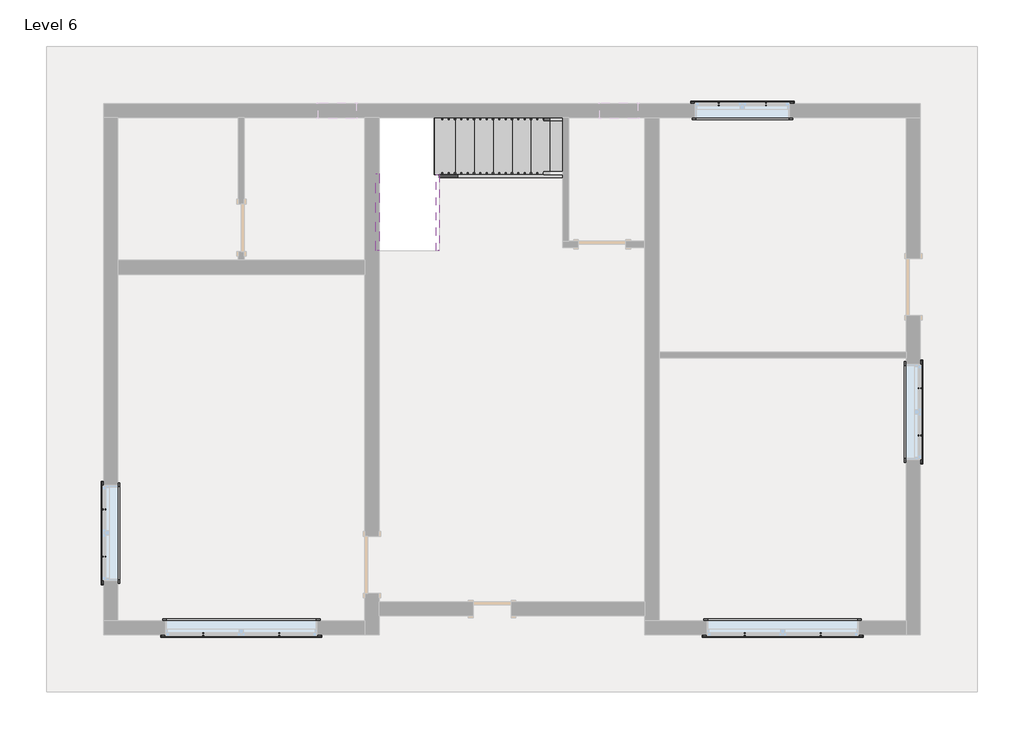
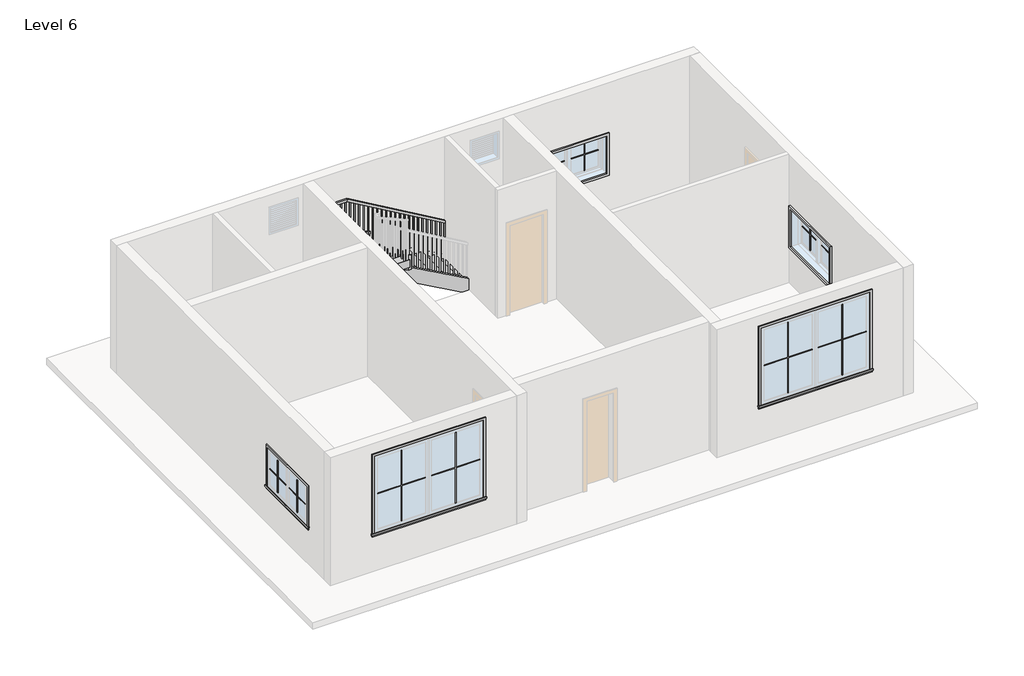
# One storey, part 2 of 2: 20 proxies, 4 members, 1 railing, 1 stair flight.
"""IFC4 building model written with IfcOpenShell, lengths in millimetres."""

from ifc_helpers import new_model, si_unit, frame, origin, place, context, project, spatial, polyline, outline, extrude, faceted_brep, transform, mapped, element, save
from components import muntin_pattern_2x2_muntin_pattern_2x2_9352d081, muntin_pattern_2x2_muntin_pattern_2x2_5c2cbe28, muntin_pattern_2x2_muntin_pattern_2x2_bb8d4d84, muntin_pattern_2x2_muntin_pattern_2x2_d03a1f3c, trim_window_exterior_flat_with_sill_979bde60, trim_window_exterior_flat_with_sill_359ed2ce, trim_window_interior_flat_picture_frame_7883d11b, trim_window_interior_flat_picture_frame_939a8053, stair_flight_d8623c0a

model = new_model("IFC4")

# Units and contexts
model_context = context("Model", 3, world=origin())
ifc_project = project(units=[si_unit("LENGTHUNIT", "METRE", prefix="MILLI")], contexts=[model_context])

# Site, building, storey
site = spatial("IfcSite", under=ifc_project)
building = spatial("IfcBuilding", under=site)
storey = spatial("IfcBuildingStorey", under=building, Name="Level 6", Elevation=15849.6)

# Proxies
placement = place(None, origin())
muntin_pattern_2x2_muntin_pattern_2x2_shape = muntin_pattern_2x2_muntin_pattern_2x2_9352d081(model_context)
element("IfcBuildingElementProxy", 1, Name="Muntin Pattern_2x2 : Muntin Pattern_2x2", ObjectType="Muntin Pattern_2x2 : Muntin Pattern_2x2", at=placement, inside=storey, context=model_context, shape_type="MappedRepresentation", body=[
    mapped(muntin_pattern_2x2_muntin_pattern_2x2_shape, transform((-7798.9165084, -1764.5743005, 16833.85), x_axis=(0.0, 1.0, 0.0), y_axis=(-1.0, 0.0, 0.0), z_axis=(0.0, 0.0, 1.0))),
])
element("IfcBuildingElementProxy", 2, Name="Muntin Pattern_2x2 : Muntin Pattern_2x2", ObjectType="Muntin Pattern_2x2 : Muntin Pattern_2x2", at=placement, inside=storey, context=model_context, shape_type="MappedRepresentation", body=[
    mapped(muntin_pattern_2x2_muntin_pattern_2x2_shape, transform((5288.4334916, 937.3506995, 16833.85), x_axis=(0.0, -1.0, 0.0), y_axis=(1.0, 0.0, 0.0), z_axis=(0.0, 0.0, 1.0))),
])
element("IfcBuildingElementProxy", 3, Name="Muntin Pattern_2x2 : Muntin Pattern_2x2", ObjectType="Muntin Pattern_2x2 : Muntin Pattern_2x2", at=placement, inside=storey, context=model_context, shape_type="MappedRepresentation", body=[
    mapped(muntin_pattern_2x2_muntin_pattern_2x2_shape, transform((2061.0459916, 5501.4131995, 16833.85), x_axis=(1.0, 0.0, 0.0), y_axis=(0.0, 1.0, 0.0), z_axis=(0.0, 0.0, 1.0))),
])
muntin_pattern_2x2_muntin_pattern_2x2_2_shape = muntin_pattern_2x2_muntin_pattern_2x2_5c2cbe28(model_context)
element("IfcBuildingElementProxy", 4, Name="Muntin Pattern_2x2 : Muntin Pattern_2x2", ObjectType="Muntin Pattern_2x2 : Muntin Pattern_2x2", at=placement, inside=storey, context=model_context, shape_type="MappedRepresentation", body=[
    mapped(muntin_pattern_2x2_muntin_pattern_2x2_2_shape, transform((-7798.9165084, -1005.7493005, 16833.85), x_axis=(0.0, -1.0, 0.0), y_axis=(1.0, 0.0, 0.0), z_axis=(0.0, 0.0, 1.0))),
])
element("IfcBuildingElementProxy", 5, Name="Muntin Pattern_2x2 : Muntin Pattern_2x2", ObjectType="Muntin Pattern_2x2 : Muntin Pattern_2x2", at=placement, inside=storey, context=model_context, shape_type="MappedRepresentation", body=[
    mapped(muntin_pattern_2x2_muntin_pattern_2x2_2_shape, transform((5288.4334916, 178.5256995, 16833.85), x_axis=(0.0, 1.0, 0.0), y_axis=(-1.0, 0.0, 0.0), z_axis=(0.0, 0.0, 1.0))),
])
element("IfcBuildingElementProxy", 6, Name="Muntin Pattern_2x2 : Muntin Pattern_2x2", ObjectType="Muntin Pattern_2x2 : Muntin Pattern_2x2", at=placement, inside=storey, context=model_context, shape_type="MappedRepresentation", body=[
    mapped(muntin_pattern_2x2_muntin_pattern_2x2_2_shape, transform((2819.8709916, 5501.4131995, 16833.85), x_axis=(-1.0, 0.0, 0.0), y_axis=(0.0, -1.0, 0.0), z_axis=(0.0, 0.0, 1.0))),
])
muntin_pattern_2x2_muntin_pattern_2x2_3_shape = muntin_pattern_2x2_muntin_pattern_2x2_bb8d4d84(model_context)
element("IfcBuildingElementProxy", 7, Name="Muntin Pattern_2x2 : Muntin Pattern_2x2", ObjectType="Muntin Pattern_2x2 : Muntin Pattern_2x2", at=placement, inside=storey, context=model_context, shape_type="MappedRepresentation", body=[
    mapped(muntin_pattern_2x2_muntin_pattern_2x2_3_shape, transform((-4990.6290084, -3013.9368005, 16833.85), x_axis=(-1.0, 0.0, 0.0), y_axis=(0.0, -1.0, 0.0), z_axis=(0.0, 0.0, 1.0))),
])
element("IfcBuildingElementProxy", 8, Name="Muntin Pattern_2x2 : Muntin Pattern_2x2", ObjectType="Muntin Pattern_2x2 : Muntin Pattern_2x2", at=placement, inside=storey, context=model_context, shape_type="MappedRepresentation", body=[
    mapped(muntin_pattern_2x2_muntin_pattern_2x2_3_shape, transform((3696.1709916, -3013.9368005, 16833.85), x_axis=(-1.0, 0.0, 0.0), y_axis=(0.0, -1.0, 0.0), z_axis=(0.0, 0.0, 1.0))),
])
muntin_pattern_2x2_muntin_pattern_2x2_4_shape = muntin_pattern_2x2_muntin_pattern_2x2_d03a1f3c(model_context)
element("IfcBuildingElementProxy", 9, Name="Muntin Pattern_2x2 : Muntin Pattern_2x2", ObjectType="Muntin Pattern_2x2 : Muntin Pattern_2x2", at=placement, inside=storey, context=model_context, shape_type="MappedRepresentation", body=[
    mapped(muntin_pattern_2x2_muntin_pattern_2x2_4_shape, transform((-6206.6540084, -3013.9368005, 16833.85), x_axis=(1.0, 0.0, 0.0), y_axis=(0.0, 1.0, 0.0), z_axis=(0.0, 0.0, 1.0))),
])
element("IfcBuildingElementProxy", 10, Name="Muntin Pattern_2x2 : Muntin Pattern_2x2", ObjectType="Muntin Pattern_2x2 : Muntin Pattern_2x2", at=placement, inside=storey, context=model_context, shape_type="MappedRepresentation", body=[
    mapped(muntin_pattern_2x2_muntin_pattern_2x2_4_shape, transform((2480.1459916, -3013.9368005, 16833.85), x_axis=(1.0, 0.0, 0.0), y_axis=(0.0, 1.0, 0.0), z_axis=(0.0, 0.0, 1.0))),
])
trim_window_exterior_flat_with_sill_shape = trim_window_exterior_flat_with_sill_979bde60(model_context)
element("IfcBuildingElementProxy", 11, Name="Trim-Window-Exterior-Flat : with Sill", ObjectType="Trim-Window-Exterior-Flat : with Sill", at=placement, inside=storey, context=model_context, shape_type="MappedRepresentation", body=[
    mapped(trim_window_exterior_flat_with_sill_shape, transform((-7808.4415084, -1385.1618005, 17678.4), x_axis=(0.0, -1.0, 0.0), y_axis=(0.0, 0.0, 1.0), z_axis=(-1.0, 0.0, 0.0))),
])
element("IfcBuildingElementProxy", 12, Name="Trim-Window-Exterior-Flat : with Sill", ObjectType="Trim-Window-Exterior-Flat : with Sill", at=placement, inside=storey, context=model_context, shape_type="MappedRepresentation", body=[
    mapped(trim_window_exterior_flat_with_sill_shape, transform((5297.9584916, 557.9381995, 17678.4), x_axis=(0.0, 1.0, 0.0), y_axis=(0.0, 0.0, 1.0), z_axis=(1.0, 0.0, 0.0))),
])
element("IfcBuildingElementProxy", 13, Name="Trim-Window-Exterior-Flat : with Sill", ObjectType="Trim-Window-Exterior-Flat : with Sill", at=placement, inside=storey, context=model_context, shape_type="MappedRepresentation", body=[
    mapped(trim_window_exterior_flat_with_sill_shape, transform((2440.4584916, 5510.9381995, 17678.4), x_axis=(-1.0, 0.0, 0.0), y_axis=(0.0, 0.0, 1.0), z_axis=(0.0, 1.0, 0.0))),
])
trim_window_exterior_flat_with_sill_2_shape = trim_window_exterior_flat_with_sill_359ed2ce(model_context)
element("IfcBuildingElementProxy", 14, Name="Trim-Window-Exterior-Flat : with Sill", ObjectType="Trim-Window-Exterior-Flat : with Sill", at=placement, inside=storey, context=model_context, shape_type="MappedRepresentation", body=[
    mapped(trim_window_exterior_flat_with_sill_2_shape, transform((-5598.6415084, -3023.4618005, 18592.8), x_axis=(1.0, 0.0, 0.0), y_axis=(0.0, 0.0, 1.0), z_axis=(0.0, -1.0, 0.0))),
])
element("IfcBuildingElementProxy", 15, Name="Trim-Window-Exterior-Flat : with Sill", ObjectType="Trim-Window-Exterior-Flat : with Sill", at=placement, inside=storey, context=model_context, shape_type="MappedRepresentation", body=[
    mapped(trim_window_exterior_flat_with_sill_2_shape, transform((3088.1584916, -3023.4618005, 18592.8), x_axis=(1.0, 0.0, 0.0), y_axis=(0.0, 0.0, 1.0), z_axis=(0.0, -1.0, 0.0))),
])
trim_window_interior_flat_picture_frame_shape = trim_window_interior_flat_picture_frame_7883d11b(model_context)
element("IfcBuildingElementProxy", 16, Name="Trim-Window-Interior-Flat : Picture Frame", ObjectType="Trim-Window-Interior-Flat : Picture Frame", at=placement, inside=storey, context=model_context, shape_type="MappedRepresentation", body=[
    mapped(trim_window_interior_flat_picture_frame_shape, transform((-7579.8415084, -1385.1618005, 17678.4), x_axis=(0.0, 1.0, 0.0), y_axis=(0.0, 0.0, 1.0), z_axis=(1.0, 0.0, 0.0))),
])
element("IfcBuildingElementProxy", 17, Name="Trim-Window-Interior-Flat : Picture Frame", ObjectType="Trim-Window-Interior-Flat : Picture Frame", at=placement, inside=storey, context=model_context, shape_type="MappedRepresentation", body=[
    mapped(trim_window_interior_flat_picture_frame_shape, transform((5069.3584916, 557.9381995, 17678.4), x_axis=(0.0, -1.0, 0.0), y_axis=(0.0, 0.0, 1.0), z_axis=(-1.0, 0.0, 0.0))),
])
element("IfcBuildingElementProxy", 18, Name="Trim-Window-Interior-Flat : Picture Frame", ObjectType="Trim-Window-Interior-Flat : Picture Frame", at=placement, inside=storey, context=model_context, shape_type="MappedRepresentation", body=[
    mapped(trim_window_interior_flat_picture_frame_shape, transform((2440.4584916, 5282.3381995, 17678.4), x_axis=(1.0, 0.0, 0.0), y_axis=(0.0, 0.0, 1.0), z_axis=(0.0, -1.0, 0.0))),
])
trim_window_interior_flat_picture_frame_2_shape = trim_window_interior_flat_picture_frame_939a8053(model_context)
element("IfcBuildingElementProxy", 19, Name="Trim-Window-Interior-Flat : Picture Frame", ObjectType="Trim-Window-Interior-Flat : Picture Frame", at=placement, inside=storey, context=model_context, shape_type="MappedRepresentation", body=[
    mapped(trim_window_interior_flat_picture_frame_2_shape, transform((-5598.6415084, -2794.8618005, 18592.8), x_axis=(-1.0, 0.0, 0.0), y_axis=(0.0, 0.0, 1.0), z_axis=(0.0, 1.0, 0.0))),
])
element("IfcBuildingElementProxy", 20, Name="Trim-Window-Interior-Flat : Picture Frame", ObjectType="Trim-Window-Interior-Flat : Picture Frame", at=placement, inside=storey, context=model_context, shape_type="MappedRepresentation", body=[
    mapped(trim_window_interior_flat_picture_frame_2_shape, transform((3088.1584916, -2794.8618005, 18592.8), x_axis=(-1.0, 0.0, 0.0), y_axis=(0.0, 0.0, 1.0), z_axis=(0.0, 1.0, 0.0))),
])

# Members
element("IfcMember", 21, ObjectType="Stringer - 2\" Width", at=placement, inside=storey, context=model_context, shape_type="SweptSolid", body=[
    extrude(outline(polyline([(15849.6, -442.4415084), (16113.6428392, -442.4415084), (17214.3095059, -2423.6415084), (16865.6308318, -2423.6415084), (15849.6, -594.7860112), (15849.6, -442.4415084)])), frame((0.0, 4317.5146777, 0.0), z_axis=(0.0, 1.0, 0.0), x_axis=(0.0, 0.0, 1.0)), (0.0, 0.0, 1.0), 50.8),
])
element("IfcMember", 22, ObjectType="Stringer - 2\" Width", at=placement, inside=storey, context=model_context, shape_type="SweptSolid", body=[
    extrude(outline(polyline([(4368.3146777, 17411.845537), (4368.3146777, 17063.2006925), (3148.7383287, 17740.4643411), (3148.7383287, 18089.1091856), (4368.3146777, 17411.845537)])), frame((-2474.4415084, 0.0, 0.0), z_axis=(1.0, 0.0, 0.0), x_axis=(0.0, 1.0, 0.0)), (0.0, 0.0, 1.0), 50.8),
])
element("IfcMember", 23, ObjectType="Stringer - 2\" Width", at=placement, inside=storey, context=model_context, shape_type="SweptSolid", body=[
    extrude(outline(polyline([(15849.6, -442.4415084), (16113.6428392, -442.4415084), (16904.2636166, -1865.5589077), (16904.2636166, -2493.1805211), (15849.6, -594.7860112), (15849.6, -442.4415084)])), frame((0.0, 5282.3381995, 0.0), z_axis=(0.0, 1.0, 0.0), x_axis=(0.0, 0.0, 1.0)), (0.0, 0.0, 1.0), 50.8),
])
element("IfcMember", 24, ObjectType="Stringer - 2\" Width", at=placement, inside=storey, context=model_context, shape_type="SweptSolid", body=[
    extrude(outline(polyline([(3758.489521, 17401.853054), (3148.7383287, 17740.4643411), (3148.7383287, 18089.1091856), (4386.3085505, 17401.853054), (3758.489521, 17401.853054)])), frame((-3439.6415084, 0.0, 0.0), z_axis=(1.0, 0.0, 0.0), x_axis=(0.0, 1.0, 0.0)), (0.0, 0.0, 1.0), 50.8),
])

# Railing
element("IfcRailing", 25, ObjectType="Handrail - Rectangular", at=placement, inside=storey, context=model_context, shape_type="SolidModel", body=[
    faceted_brep([(-442.4415084, 5231.5381995, 16933.3333333), (-442.4415084, 5231.5381995, 16874.5219871), (-442.4415084, 5282.3381995, 16874.5219871), (-442.4415084, 5282.3381995, 16933.3333333), (-2641.0608886, 5231.5381995, 18215.8613051), (-2654.794625, 5231.5381995, 18165.0613051), (-2654.794625, 5282.3381995, 18165.0613051), (-2641.0608886, 5282.3381995, 18215.8613051), (-3338.0415084, 5231.5381995, 18215.8613051), (-3338.0415084, 5231.5381995, 18165.0613051), (-3388.8415084, 5282.3381995, 18165.0613051), (-3388.8415084, 5282.3381995, 18215.8613051), (-3338.0415084, 4498.2044111, 18215.8613051), (-3338.0415084, 4485.04436, 18165.0613051), (-3388.8415084, 4485.04436, 18165.0613051), (-3388.8415084, 4498.2044111, 18215.8613051), (-3338.0415084, 3148.7383287, 18965.3333333), (-3388.8415084, 3148.7383287, 18965.3333333), (-3388.8415084, 3148.7383287, 18907.22445), (-3338.0415084, 3148.7383287, 18907.22445)], [[[0, 1, 2, 3]], [[1, 0, 4, 5]], [[2, 1, 5, 6]], [[3, 2, 6, 7]], [[0, 3, 7, 4]], [[5, 4, 8, 9]], [[6, 5, 9, 10]], [[7, 6, 10, 11]], [[4, 7, 11, 8]], [[9, 8, 12, 13]], [[10, 9, 13, 14]], [[11, 10, 14, 15]], [[8, 11, 15, 12]], [[16, 17, 18, 19]], [[13, 12, 16, 19]], [[14, 13, 19, 18]], [[15, 14, 18, 17]], [[12, 15, 17, 16]]]),
    extrude(outline(polyline([(3215.4131995, 18870.1942858), (3234.4631995, 18859.6142183), (3234.4631995, 17881.6), (3215.4131995, 17881.6), (3215.4131995, 18870.1942858)])), frame((-3372.9665084, 0.0, 0.0), z_axis=(1.0, 0.0, 0.0), x_axis=(0.0, 1.0, 0.0)), (0.0, 0.0, 1.0), 19.05),
    extrude(outline(polyline([(3317.0131995, 18813.9240232), (3336.0631995, 18803.3439558), (3336.0631995, 17881.6), (3317.0131995, 17881.6), (3317.0131995, 18813.9240232)])), frame((-3372.9665084, 0.0, 0.0), z_axis=(1.0, 0.0, 0.0), x_axis=(0.0, 1.0, 0.0)), (0.0, 0.0, 1.0), 19.05),
    extrude(outline(polyline([(3418.6131995, 18757.4969969), (3437.6631995, 18746.9169295), (3437.6631995, 17881.6), (3418.6131995, 17881.6), (3418.6131995, 18757.4969969)])), frame((-3372.9665084, 0.0, 0.0), z_axis=(1.0, 0.0, 0.0), x_axis=(0.0, 1.0, 0.0)), (0.0, 0.0, 1.0), 19.05),
    extrude(outline(polyline([(3520.2131995, 18701.0699707), (3539.2631995, 18690.4899033), (3539.2631995, 17712.2666667), (3520.2131995, 17712.2666667), (3520.2131995, 18701.0699707)])), frame((-3372.9665084, 0.0, 0.0), z_axis=(1.0, 0.0, 0.0), x_axis=(0.0, 1.0, 0.0)), (0.0, 0.0, 1.0), 19.05),
    extrude(outline(polyline([(3621.8131995, 18644.5906899), (3640.8631995, 18634.0106224), (3640.8631995, 17712.2666667), (3621.8131995, 17712.2666667), (3621.8131995, 18644.5906899)])), frame((-3372.9665084, 0.0, 0.0), z_axis=(1.0, 0.0, 0.0), x_axis=(0.0, 1.0, 0.0)), (0.0, 0.0, 1.0), 19.05),
    extrude(outline(polyline([(3723.4131995, 18588.1636636), (3742.4631995, 18577.5835962), (3742.4631995, 17712.2666667), (3723.4131995, 17712.2666667), (3723.4131995, 18588.1636636)])), frame((-3372.9665084, 0.0, 0.0), z_axis=(1.0, 0.0, 0.0), x_axis=(0.0, 1.0, 0.0)), (0.0, 0.0, 1.0), 19.05),
    extrude(outline(polyline([(3825.0131995, 18531.7366374), (3844.0631995, 18521.1565699), (3844.0631995, 17542.9333333), (3825.0131995, 17542.9333333), (3825.0131995, 18531.7366374)])), frame((-3372.9665084, 0.0, 0.0), z_axis=(1.0, 0.0, 0.0), x_axis=(0.0, 1.0, 0.0)), (0.0, 0.0, 1.0), 19.05),
    extrude(outline(polyline([(3926.6131995, 18475.2573565), (3945.6631995, 18464.6772891), (3945.6631995, 17542.9333333), (3926.6131995, 17542.9333333), (3926.6131995, 18475.2573565)])), frame((-3372.9665084, 0.0, 0.0), z_axis=(1.0, 0.0, 0.0), x_axis=(0.0, 1.0, 0.0)), (0.0, 0.0, 1.0), 19.05),
    extrude(outline(polyline([(4028.2131995, 18418.8303303), (4047.2631995, 18408.2502629), (4047.2631995, 17542.9333333), (4028.2131995, 17542.9333333), (4028.2131995, 18418.8303303)])), frame((-3372.9665084, 0.0, 0.0), z_axis=(1.0, 0.0, 0.0), x_axis=(0.0, 1.0, 0.0)), (0.0, 0.0, 1.0), 19.05),
    extrude(outline(polyline([(4129.8131995, 18362.403304), (4148.8631995, 18351.8232366), (4148.8631995, 17373.6), (4129.8131995, 17373.6), (4129.8131995, 18362.403304)])), frame((-3372.9665084, 0.0, 0.0), z_axis=(1.0, 0.0, 0.0), x_axis=(0.0, 1.0, 0.0)), (0.0, 0.0, 1.0), 19.05),
    extrude(outline(polyline([(4231.4131995, 18305.9240232), (4250.4631995, 18295.3439558), (4250.4631995, 17373.6), (4231.4131995, 17373.6), (4231.4131995, 18305.9240232)])), frame((-3372.9665084, 0.0, 0.0), z_axis=(1.0, 0.0, 0.0), x_axis=(0.0, 1.0, 0.0)), (0.0, 0.0, 1.0), 19.05),
    extrude(outline(polyline([(4333.0131995, 18249.4969969), (4352.0631995, 18238.9169295), (4352.0631995, 17373.6), (4333.0131995, 17373.6), (4333.0131995, 18249.4969969)])), frame((-3372.9665084, 0.0, 0.0), z_axis=(1.0, 0.0, 0.0), x_axis=(0.0, 1.0, 0.0)), (0.0, 0.0, 1.0), 19.05),
    extrude(outline(polyline([(4434.6131995, 18193.0699707), (4453.6631995, 18182.4899033), (4453.6631995, 17204.2666667), (4434.6131995, 17204.2666667), (4434.6131995, 18193.0699707)])), frame((-3372.9665084, 0.0, 0.0), z_axis=(1.0, 0.0, 0.0), x_axis=(0.0, 1.0, 0.0)), (0.0, 0.0, 1.0), 19.05),
    extrude(outline(polyline([(-3372.9665084, 4555.2631995), (-3353.9165084, 4555.2631995), (-3353.9165084, 4536.2131995), (-3372.9665084, 4536.2131995), (-3372.9665084, 4555.2631995)])), frame((0.0, 0.0, 17204.2666667), z_axis=(0.0, 0.0, 1.0), x_axis=(1.0, 0.0, 0.0)), (0.0, 0.0, 1.0), 960.7946385),
    extrude(outline(polyline([(-3372.9665084, 4656.8631995), (-3353.9165084, 4656.8631995), (-3353.9165084, 4637.8131995), (-3372.9665084, 4637.8131995), (-3372.9665084, 4656.8631995)])), frame((0.0, 0.0, 17204.2666667), z_axis=(0.0, 0.0, 1.0), x_axis=(1.0, 0.0, 0.0)), (0.0, 0.0, 1.0), 960.7946385),
    extrude(outline(polyline([(-3372.9665084, 4758.4631995), (-3353.9165084, 4758.4631995), (-3353.9165084, 4739.4131995), (-3372.9665084, 4739.4131995), (-3372.9665084, 4758.4631995)])), frame((0.0, 0.0, 17204.2666667), z_axis=(0.0, 0.0, 1.0), x_axis=(1.0, 0.0, 0.0)), (0.0, 0.0, 1.0), 960.7946385),
    extrude(outline(polyline([(-3372.9665084, 4860.0631995), (-3353.9165084, 4860.0631995), (-3353.9165084, 4841.0131995), (-3372.9665084, 4841.0131995), (-3372.9665084, 4860.0631995)])), frame((0.0, 0.0, 17204.2666667), z_axis=(0.0, 0.0, 1.0), x_axis=(1.0, 0.0, 0.0)), (0.0, 0.0, 1.0), 960.7946385),
    extrude(outline(polyline([(-3372.9665084, 4961.6631995), (-3353.9165084, 4961.6631995), (-3353.9165084, 4942.6131995), (-3372.9665084, 4942.6131995), (-3372.9665084, 4961.6631995)])), frame((0.0, 0.0, 17204.2666667), z_axis=(0.0, 0.0, 1.0), x_axis=(1.0, 0.0, 0.0)), (0.0, 0.0, 1.0), 960.7946385),
    extrude(outline(polyline([(-3372.9665084, 5063.2631995), (-3353.9165084, 5063.2631995), (-3353.9165084, 5044.2131995), (-3372.9665084, 5044.2131995), (-3372.9665084, 5063.2631995)])), frame((0.0, 0.0, 17204.2666667), z_axis=(0.0, 0.0, 1.0), x_axis=(1.0, 0.0, 0.0)), (0.0, 0.0, 1.0), 960.7946385),
    extrude(outline(polyline([(-3372.9665084, 5164.8631995), (-3353.9165084, 5164.8631995), (-3353.9165084, 5145.8131995), (-3372.9665084, 5145.8131995), (-3372.9665084, 5164.8631995)])), frame((0.0, 0.0, 17204.2666667), z_axis=(0.0, 0.0, 1.0), x_axis=(1.0, 0.0, 0.0)), (0.0, 0.0, 1.0), 960.7946385),
    extrude(outline(polyline([(-3277.7165084, 5266.4631995), (-3277.7165084, 5247.4131995), (-3296.7665084, 5247.4131995), (-3296.7665084, 5266.4631995), (-3277.7165084, 5266.4631995)])), frame((0.0, 0.0, 17204.2666667), z_axis=(0.0, 0.0, 1.0), x_axis=(1.0, 0.0, 0.0)), (0.0, 0.0, 1.0), 960.7946385),
    extrude(outline(polyline([(-3176.1165084, 5266.4631995), (-3176.1165084, 5247.4131995), (-3195.1665084, 5247.4131995), (-3195.1665084, 5266.4631995), (-3176.1165084, 5266.4631995)])), frame((0.0, 0.0, 17204.2666667), z_axis=(0.0, 0.0, 1.0), x_axis=(1.0, 0.0, 0.0)), (0.0, 0.0, 1.0), 960.7946385),
    extrude(outline(polyline([(-3074.5165084, 5266.4631995), (-3074.5165084, 5247.4131995), (-3093.5665084, 5247.4131995), (-3093.5665084, 5266.4631995), (-3074.5165084, 5266.4631995)])), frame((0.0, 0.0, 17204.2666667), z_axis=(0.0, 0.0, 1.0), x_axis=(1.0, 0.0, 0.0)), (0.0, 0.0, 1.0), 960.7946385),
    extrude(outline(polyline([(-2972.9165084, 5266.4631995), (-2972.9165084, 5247.4131995), (-2991.9665084, 5247.4131995), (-2991.9665084, 5266.4631995), (-2972.9165084, 5266.4631995)])), frame((0.0, 0.0, 17204.2666667), z_axis=(0.0, 0.0, 1.0), x_axis=(1.0, 0.0, 0.0)), (0.0, 0.0, 1.0), 960.7946385),
    extrude(outline(polyline([(-2871.3165084, 5266.4631995), (-2871.3165084, 5247.4131995), (-2890.3665084, 5247.4131995), (-2890.3665084, 5266.4631995), (-2871.3165084, 5266.4631995)])), frame((0.0, 0.0, 17204.2666667), z_axis=(0.0, 0.0, 1.0), x_axis=(1.0, 0.0, 0.0)), (0.0, 0.0, 1.0), 960.7946385),
    extrude(outline(polyline([(-2769.7165084, 5266.4631995), (-2769.7165084, 5247.4131995), (-2788.7665084, 5247.4131995), (-2788.7665084, 5266.4631995), (-2769.7165084, 5266.4631995)])), frame((0.0, 0.0, 17204.2666667), z_axis=(0.0, 0.0, 1.0), x_axis=(1.0, 0.0, 0.0)), (0.0, 0.0, 1.0), 960.7946385),
    extrude(outline(polyline([(-2668.1165084, 5266.4631995), (-2668.1165084, 5247.4131995), (-2687.1665084, 5247.4131995), (-2687.1665084, 5266.4631995), (-2668.1165084, 5266.4631995)])), frame((0.0, 0.0, 17204.2666667), z_axis=(0.0, 0.0, 1.0), x_axis=(1.0, 0.0, 0.0)), (0.0, 0.0, 1.0), 960.7946385),
    extrude(outline(polyline([(18113.5657371, -2566.5165084), (18124.6782371, -2585.5665084), (17204.2666667, -2585.5665084), (17204.2666667, -2566.5165084), (18113.5657371, -2566.5165084)])), frame((0.0, 5247.4131995, 0.0), z_axis=(0.0, 1.0, 0.0), x_axis=(0.0, 0.0, 1.0)), (0.0, 0.0, 1.0), 19.05),
    extrude(outline(polyline([(18054.2990704, -2464.9165084), (18065.4115704, -2483.9665084), (17204.2666667, -2483.9665084), (17204.2666667, -2464.9165084), (18054.2990704, -2464.9165084)])), frame((0.0, 5247.4131995, 0.0), z_axis=(0.0, 1.0, 0.0), x_axis=(0.0, 0.0, 1.0)), (0.0, 0.0, 1.0), 19.05),
    extrude(outline(polyline([(17995.0324038, -2363.3165084), (18006.1449038, -2382.3665084), (17034.9333333, -2382.3665084), (17034.9333333, -2363.3165084), (17995.0324038, -2363.3165084)])), frame((0.0, 5247.4131995, 0.0), z_axis=(0.0, 1.0, 0.0), x_axis=(0.0, 0.0, 1.0)), (0.0, 0.0, 1.0), 19.05),
    extrude(outline(polyline([(17935.7657371, -2261.7165084), (17946.8782371, -2280.7665084), (17034.9333333, -2280.7665084), (17034.9333333, -2261.7165084), (17935.7657371, -2261.7165084)])), frame((0.0, 5247.4131995, 0.0), z_axis=(0.0, 1.0, 0.0), x_axis=(0.0, 0.0, 1.0)), (0.0, 0.0, 1.0), 19.05),
    extrude(outline(polyline([(17876.4990704, -2160.1165084), (17887.6115704, -2179.1665084), (17034.9333333, -2179.1665084), (17034.9333333, -2160.1165084), (17876.4990704, -2160.1165084)])), frame((0.0, 5247.4131995, 0.0), z_axis=(0.0, 1.0, 0.0), x_axis=(0.0, 0.0, 1.0)), (0.0, 0.0, 1.0), 19.05),
    extrude(outline(polyline([(17817.2324038, -2058.5165084), (17828.3449038, -2077.5665084), (16865.6, -2077.5665084), (16865.6, -2058.5165084), (17817.2324038, -2058.5165084)])), frame((0.0, 5247.4131995, 0.0), z_axis=(0.0, 1.0, 0.0), x_axis=(0.0, 0.0, 1.0)), (0.0, 0.0, 1.0), 19.05),
    extrude(outline(polyline([(17757.9657371, -1956.9165084), (17769.0782371, -1975.9665084), (16865.6, -1975.9665084), (16865.6, -1956.9165084), (17757.9657371, -1956.9165084)])), frame((0.0, 5247.4131995, 0.0), z_axis=(0.0, 1.0, 0.0), x_axis=(0.0, 0.0, 1.0)), (0.0, 0.0, 1.0), 19.05),
    extrude(outline(polyline([(17698.6990704, -1855.3165084), (17709.8115704, -1874.3665084), (16865.6, -1874.3665084), (16865.6, -1855.3165084), (17698.6990704, -1855.3165084)])), frame((0.0, 5247.4131995, 0.0), z_axis=(0.0, 1.0, 0.0), x_axis=(0.0, 0.0, 1.0)), (0.0, 0.0, 1.0), 19.05),
    extrude(outline(polyline([(17639.4324038, -1753.7165084), (17650.5449038, -1772.7665084), (16696.2666667, -1772.7665084), (16696.2666667, -1753.7165084), (17639.4324038, -1753.7165084)])), frame((0.0, 5247.4131995, 0.0), z_axis=(0.0, 1.0, 0.0), x_axis=(0.0, 0.0, 1.0)), (0.0, 0.0, 1.0), 19.05),
    extrude(outline(polyline([(17580.1657371, -1652.1165084), (17591.2782371, -1671.1665084), (16696.2666667, -1671.1665084), (16696.2666667, -1652.1165084), (17580.1657371, -1652.1165084)])), frame((0.0, 5247.4131995, 0.0), z_axis=(0.0, 1.0, 0.0), x_axis=(0.0, 0.0, 1.0)), (0.0, 0.0, 1.0), 19.05),
    extrude(outline(polyline([(17520.8990704, -1550.5165084), (17532.0115704, -1569.5665084), (16696.2666667, -1569.5665084), (16696.2666667, -1550.5165084), (17520.8990704, -1550.5165084)])), frame((0.0, 5247.4131995, 0.0), z_axis=(0.0, 1.0, 0.0), x_axis=(0.0, 0.0, 1.0)), (0.0, 0.0, 1.0), 19.05),
    extrude(outline(polyline([(17461.6324038, -1448.9165084), (17472.7449038, -1467.9665084), (16526.9333333, -1467.9665084), (16526.9333333, -1448.9165084), (17461.6324038, -1448.9165084)])), frame((0.0, 5247.4131995, 0.0), z_axis=(0.0, 1.0, 0.0), x_axis=(0.0, 0.0, 1.0)), (0.0, 0.0, 1.0), 19.05),
    extrude(outline(polyline([(17402.3657371, -1347.3165084), (17413.4782371, -1366.3665084), (16526.9333333, -1366.3665084), (16526.9333333, -1347.3165084), (17402.3657371, -1347.3165084)])), frame((0.0, 5247.4131995, 0.0), z_axis=(0.0, 1.0, 0.0), x_axis=(0.0, 0.0, 1.0)), (0.0, 0.0, 1.0), 19.05),
    extrude(outline(polyline([(17343.0990704, -1245.7165084), (17354.2115704, -1264.7665084), (16526.9333333, -1264.7665084), (16526.9333333, -1245.7165084), (17343.0990704, -1245.7165084)])), frame((0.0, 5247.4131995, 0.0), z_axis=(0.0, 1.0, 0.0), x_axis=(0.0, 0.0, 1.0)), (0.0, 0.0, 1.0), 19.05),
    extrude(outline(polyline([(17283.8324038, -1144.1165084), (17294.9449038, -1163.1665084), (16357.6, -1163.1665084), (16357.6, -1144.1165084), (17283.8324038, -1144.1165084)])), frame((0.0, 5247.4131995, 0.0), z_axis=(0.0, 1.0, 0.0), x_axis=(0.0, 0.0, 1.0)), (0.0, 0.0, 1.0), 19.05),
    extrude(outline(polyline([(17224.5657371, -1042.5165084), (17235.6782371, -1061.5665084), (16357.6, -1061.5665084), (16357.6, -1042.5165084), (17224.5657371, -1042.5165084)])), frame((0.0, 5247.4131995, 0.0), z_axis=(0.0, 1.0, 0.0), x_axis=(0.0, 0.0, 1.0)), (0.0, 0.0, 1.0), 19.05),
    extrude(outline(polyline([(17165.2990704, -940.9165084), (17176.4115704, -959.9665084), (16357.6, -959.9665084), (16357.6, -940.9165084), (17165.2990704, -940.9165084)])), frame((0.0, 5247.4131995, 0.0), z_axis=(0.0, 1.0, 0.0), x_axis=(0.0, 0.0, 1.0)), (0.0, 0.0, 1.0), 19.05),
    extrude(outline(polyline([(17106.0324038, -839.3165084), (17117.1449038, -858.3665084), (16188.2666667, -858.3665084), (16188.2666667, -839.3165084), (17106.0324038, -839.3165084)])), frame((0.0, 5247.4131995, 0.0), z_axis=(0.0, 1.0, 0.0), x_axis=(0.0, 0.0, 1.0)), (0.0, 0.0, 1.0), 19.05),
    extrude(outline(polyline([(17046.7657371, -737.7165084), (17057.8782371, -756.7665084), (16188.2666667, -756.7665084), (16188.2666667, -737.7165084), (17046.7657371, -737.7165084)])), frame((0.0, 5247.4131995, 0.0), z_axis=(0.0, 1.0, 0.0), x_axis=(0.0, 0.0, 1.0)), (0.0, 0.0, 1.0), 19.05),
    extrude(outline(polyline([(16987.4990704, -636.1165084), (16998.6115704, -655.1665084), (16188.2666667, -655.1665084), (16188.2666667, -636.1165084), (16987.4990704, -636.1165084)])), frame((0.0, 5247.4131995, 0.0), z_axis=(0.0, 1.0, 0.0), x_axis=(0.0, 0.0, 1.0)), (0.0, 0.0, 1.0), 19.05),
    extrude(outline(polyline([(16928.2324038, -534.5165084), (16939.3449038, -553.5665084), (16018.9333333, -553.5665084), (16018.9333333, -534.5165084), (16928.2324038, -534.5165084)])), frame((0.0, 5247.4131995, 0.0), z_axis=(0.0, 1.0, 0.0), x_axis=(0.0, 0.0, 1.0)), (0.0, 0.0, 1.0), 19.05),
    extrude(outline(polyline([(-3353.9165084, 5266.4631995), (-3353.9165084, 5247.4131995), (-3372.9665084, 5247.4131995), (-3372.9665084, 5266.4631995), (-3353.9165084, 5266.4631995)])), frame((0.0, 0.0, 17204.2666667), z_axis=(0.0, 0.0, 1.0), x_axis=(1.0, 0.0, 0.0)), (0.0, 0.0, 1.0), 960.7946385),
    extrude(outline(polyline([(3148.7383287, 18907.22445), (3167.7883287, 18896.6443826), (3167.7883287, 17881.6), (3148.7383287, 17881.6), (3148.7383287, 18907.22445)])), frame((-3372.9665084, 0.0, 0.0), z_axis=(1.0, 0.0, 0.0), x_axis=(0.0, 1.0, 0.0)), (0.0, 0.0, 1.0), 19.05),
    extrude(outline(polyline([(16874.5219871, -442.4415084), (16885.6344871, -461.4915084), (16018.9333333, -461.4915084), (16018.9333333, -442.4415084), (16874.5219871, -442.4415084)])), frame((0.0, 5247.4131995, 0.0), z_axis=(0.0, 1.0, 0.0), x_axis=(0.0, 0.0, 1.0)), (0.0, 0.0, 1.0), 19.05),
])

# Stair flight
stair_flight_shape = stair_flight_d8623c0a(model_context)
element("IfcStairFlight", 26, ObjectType="2\" Tread 1\" Nosing 1/4\" Riser", at=placement, inside=storey, context=model_context, shape_type="MappedRepresentation", body=[
    mapped(stair_flight_shape, transform((0.0, 0.0, 0.0), x_axis=(1.0, 0.0, 0.0), y_axis=(0.0, 1.0, 0.0), z_axis=(0.0, 0.0, 1.0))),
])

save(model, "model.ifc")

# Revit data of these elements
# Type "Muntin Pattern_2x2 : Muntin Pattern_2x2"
#   Width [instance default] = 4' - 0"
#   Thickness = 0' - 0 1/2"
#   Height [instance default] = 4' - 0"
#   Distance = 0' - 0 3/4"
#   Interior Material [instance default] = none
#   Exterior Material [instance default] = none
#   Default Elevation = 0
# Type "Trim-Window-Exterior-Flat : with Sill"
#   Trim Width = 0' - 2 1/4"
#   Trim Thickness_Picture Frame = 0' - 1 1/4"
#   Trim Thickness_with Sill = 0' - 0 3/4"
#   Sill Thickness = 0' - 1 1/4"
#   Opening Width [instance default] = 2' - 0"
#   Opening Height [instance default] = 3' - 0"
#   Default Elevation = 4' - 0"
#   Sill = yes
#   Picture Frame = no
#   Trim Material [instance default] = none
# Type "Trim-Window-Interior-Flat : Picture Frame"
#   Trim Thickness_Picture Frame = 0' - 1 1/4"
#   Trim Width = 0' - 2 1/4"
#   Trim Thickness_with Sill = 0' - 0 3/4"
#   Sill Thickness = 0' - 1 1/4"
#   Opening Width [instance default] = 2' - 0"
#   Opening Height [instance default] = 3' - 0"
#   Default Elevation = 4' - 0"
#   Sill = no
#   Picture Frame = yes
#   Trim Material [instance default] = none
# Type "Handrail - Rectangular"
#   Assembly Code = "C2010400"
#   built-in parameter 1008612 = 0.0416667 (stored number, unit not read)
#   built-in parameter 1008611 = 0.0416667 (stored number, unit not read)
#   built-in parameter 1008609 = 0.333333 (stored number, unit not read)
#   built-in parameter 1008604 = 0.166667 (stored number, unit not read)
#   built-in parameter 1008603 = 0.166667 (stored number, unit not read)
#   Railing Height = 3' - 0"
#   built-in parameter 1008630 = 2
#   built-in parameter 1008610 = 2
#   built-in parameter 1008618 = Baluster - Square : 3/4"
# Elements 1, 2, 3, 4, 5, 6 (IfcBuildingElementProxy, "Muntin Pattern_2x2 : Muntin Pattern_2x2")
#   Width = 2' - 0 5/8"
#   Height = 2' - 6 1/2"
#   Interior Material = Wood - Stained
#   Exterior Material = Clad - White
#   Phase Created = New Construction
#   Materials on its faces: "Clad - White", "Wood - Stained"
# Elements 7, 8, 9, 10 (IfcBuildingElementProxy, "Muntin Pattern_2x2 : Muntin Pattern_2x2")
#   Width = 3' - 6 5/8"
#   Height = 5' - 6 1/2"
#   Interior Material = Wood - Stained
#   Exterior Material = Clad - White
#   Phase Created = New Construction
#   Materials on its faces: "Clad - White", "Wood - Stained"
# Elements 11, 12, 13 (IfcBuildingElementProxy, "Trim-Window-Exterior-Flat : with Sill")
#   Opening Width = 5' - 0"
#   Opening Height = 3' - 0"
#   Trim Material = Clad - White
#   Phase Created = New Construction
#   Materials on its faces: "Clad - White"
# Elements 14, 15 (IfcBuildingElementProxy, "Trim-Window-Exterior-Flat : with Sill")
#   Opening Width = 8' - 0"
#   Opening Height = 6' - 0"
#   Trim Material = Clad - White
#   Phase Created = New Construction
#   Materials on its faces: "Clad - White"
# Elements 16, 17, 18 (IfcBuildingElementProxy, "Trim-Window-Interior-Flat : Picture Frame")
#   Opening Width = 5' - 0"
#   Opening Height = 3' - 0"
#   Trim Material = Wood - Stained
#   Phase Created = New Construction
#   Materials on its faces: "Wood - Stained"
# Elements 19, 20 (IfcBuildingElementProxy, "Trim-Window-Interior-Flat : Picture Frame")
#   Opening Width = 8' - 0"
#   Opening Height = 6' - 0"
#   Trim Material = Wood - Stained
#   Phase Created = New Construction
#   Materials on its faces: "Wood - Stained"
# Elements 21, 22, 23, 24 (IfcMember, "Stringer - 2\" Width")
#   Phase Created = New Construction
# Element 25 (IfcRailing, "Handrail - Rectangular")
#   Phase Created = New Construction
# Element 26 (IfcStairFlight, "2\" Tread 1\" Nosing 1/4\" Riser")
#   Phase Created = New Construction
# Materials
#   "Clad - White": class "Wood", colour RGB 242 242 238, transparency 0, Cost = 0
#   "Wood - Stained": class "Wood", colour RGB 224 178 126, transparency 0, Cost = 0
